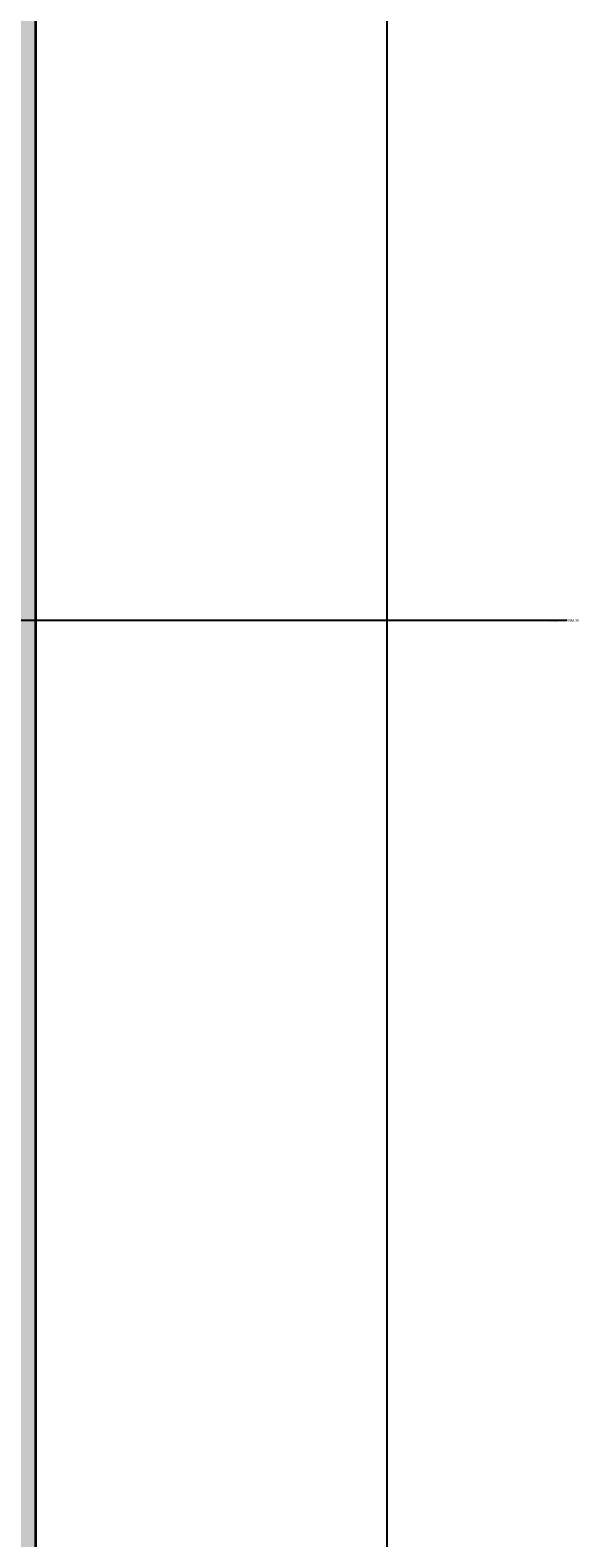
# Model space of a CAD drawing. Units: inches. Extents: x 3024 to 3952, y 1308 to 1863.
# Tile 20 of 29: x 3469 to 3510, y 1449 to 1559. Entities that reach past the tile are written whole.
import ezdxf

# ---------------------------------------------------------------- set-up
doc = ezdxf.new("R2010")
doc.units = ezdxf.units.IN
doc.layers.add('A-ANNO-DIMS', color=2, linetype='Continuous', lineweight=18)
doc.layers.add('A-WALL', color=7, linetype='Continuous', lineweight=35)
doc.layers.add('A-WALL-PATT', color=254, linetype='Continuous', lineweight=13, true_color=0xcecce6)
doc.styles.get("Standard").update_dxf_attribs({"font": 'arial.ttf'})
doc.dimstyles.get("Standard").update_dxf_attribs({"dimtxt": 0.18, "dimasz": 0.18, "dimexe": 0.18, "dimexo": 0.0625, "dimgap": 0.09, "dimtad": 0, "dimtih": 1, "dimtoh": 1, "dimdec": 4, "dimzin": 0, "dimdsep": 46, "dimtxsty": 'Standard', "dimcen": 0.09, "dimadec": 0, "dimazin": 0, "dimtfac": 1, "dimtdec": 4, "dimtofl": 0, "dimtmove": 0, "dimatfit": 3, "dimfxl": 1, "dimtolj": 1, "dimtzin": 0, "dimarcsym": 0})

# ---------------------------------------------------------------- blocks, each defined once
blk = doc.blocks.new('*D37')
at = {"layer": 'A-ANNO-DIMS', "color": 0, "lineweight": -2, "transparency": 16777216}
for p, q in [((3469.83, 1787.61), (3495.72, 1787.61)), ((3495.54, 1787.43), (3495.54, 1567.91)), ((3495.54, 1348.03), (3495.54, 1567.54)), ((3469.83, 1347.85), (3495.72, 1347.85))]:
    blk.add_line(p, q, dxfattribs=at)
at = {"layer": 'A-ANNO-DIMS', "color": 0, "transparency": 16777216}
for points in [[(3495.51, 1787.43), (3495.57, 1787.43), (3495.54, 1787.61)], [(3495.51, 1348.03), (3495.57, 1348.03), (3495.54, 1347.85)]]:
    blk.add_solid(points, dxfattribs=at)
at = {"layer": 'Defpoints', "color": 0, "transparency": 16777216}
for p in [(3469.76, 1787.61), (3495.54, 1787.61), (3469.76, 1347.85)]:
    blk.add_point(p, dxfattribs=at)
at = {"layer": 'A-ANNO-DIMS', "color": 0, "transparency": 16777216, "insert": (3495.54, 1567.73), "char_height": 0.18, "attachment_point": 5}
blk.add_mtext('\\A1;439.8', dxfattribs=at)
blk = doc.blocks.new('*D104')
at = {"layer": 'A-ANNO-DIMS', "color": 0, "lineweight": -2, "transparency": 16777216}
for p, q in [((3360.65, 1515.79), (3360.83, 1515.79)), ((3360.74, 1515.7), (3360.74, 1515.88)), ((3507.36, 1515.79), (3452.55, 1515.79))]:
    blk.add_line(p, q, dxfattribs=at)
at = {"layer": 'A-ANNO-DIMS', "color": 0, "transparency": 16777216}
blk.add_solid([(3452.55, 1515.82), (3452.55, 1515.76), (3452.37, 1515.79)], dxfattribs=at)
at = {"layer": 'Defpoints', "color": 0, "transparency": 16777216}
for p in [(3360.74, 1515.79), (3452.37, 1515.79)]:
    blk.add_point(p, dxfattribs=at)
at = {"layer": 'A-ANNO-DIMS', "color": 0, "transparency": 16777216, "insert": (3507.83, 1515.79), "char_height": 0.18, "attachment_point": 5}
blk.add_mtext('\\A1;R91.64', dxfattribs=at)
blk = doc.blocks.new('*D105')
at = {"layer": 'A-ANNO-DIMS', "color": 0, "lineweight": -2, "transparency": 16777216}
for p, q in [((3370.44, 1515.79), (3370.62, 1515.79)), ((3370.53, 1515.7), (3370.53, 1515.88)), ((3508.74, 1515.79), (3457.09, 1515.79))]:
    blk.add_line(p, q, dxfattribs=at)
at = {"layer": 'A-ANNO-DIMS', "color": 0, "transparency": 16777216}
blk.add_solid([(3457.09, 1515.82), (3457.09, 1515.76), (3456.91, 1515.79)], dxfattribs=at)
at = {"layer": 'Defpoints', "color": 0, "transparency": 16777216}
for p in [(3370.53, 1515.79), (3456.91, 1515.79)]:
    blk.add_point(p, dxfattribs=at)
at = {"layer": 'A-ANNO-DIMS', "color": 0, "transparency": 16777216, "insert": (3509.22, 1515.79), "char_height": 0.18, "attachment_point": 5}
blk.add_mtext('\\A1;R86.38', dxfattribs=at)

msp = doc.modelspace()

# ---------------------------------------------------------------- hatches: boundary and pattern name
at = {"layer": 'A-WALL-PATT'}
h = msp.add_hatch(color=256, dxfattribs=at)
h.dxf.hatch_style = 1
h.paths.add_polyline_path([(3106.764, 1778.6064), (3140.5977, 1778.6064), (3140.5977, 1781.8824), (3140.5977, 1784.6), (3140.5977, 1787.6064), (3097.764, 1787.6064), (3097.764, 1590.213), (3101.04, 1590.213), (3103.7576, 1590.213), (3106.764, 1590.213)])
h.paths.add_polyline_path([(3253.5314, 1781.8824), (3253.5314, 1784.6), (3253.5314, 1787.6064), (3194.6826, 1787.6064), (3194.6826, 1785.0146), (3194.6826, 1784.6), (3194.6826, 1781.8824), (3194.6826, 1778.6064), (3253.5314, 1778.6064)])
h.paths.add_polyline_path([(3333.856, 1782.2838), (3333.856, 1784.7474), (3333.856, 1787.6064), (3272.0523, 1787.6064), (3272.0523, 1785.0146), (3272.0523, 1784.6), (3272.0523, 1781.8824), (3272.0523, 1778.6064), (3333.856, 1778.6064)])
h.paths.add_polyline_path([(3428.8344, 1784.6), (3428.8344, 1787.6064), (3378.3947, 1787.6064), (3378.3947, 1784.7474), (3378.3947, 1782.2838), (3378.3947, 1778.6064), (3428.8344, 1778.6064), (3428.8344, 1781.8824)], flags=17)
h.paths.add_polyline_path([(3469.764, 1787.6064), (3451.9386, 1787.6064), (3451.9386, 1785.0146), (3451.9386, 1784.6), (3451.9386, 1781.8824), (3451.9386, 1778.6064), (3460.764, 1778.6064), (3460.764, 1353.8452), (3277.764, 1353.8452), (3277.764, 1347.8452), (3469.764, 1347.8452), (3469.764, 1353.8452)])
h.paths.add_polyline_path([(3106.764, 1571.6922), (3104.1722, 1571.6922), (3103.7576, 1571.6922), (3101.04, 1571.6922), (3097.764, 1571.6922), (3097.764, 1347.8452), (3148.7271, 1347.8452), (3148.7271, 1351.1212), (3148.7271, 1353.8388), (3148.7271, 1356.8452), (3106.764, 1356.8452)])
h.paths.add_polyline_path([(3277.764, 1532.6064), (3262.7605, 1532.6064), (3262.7605, 1582.9359), (3256.7605, 1582.9359), (3256.7605, 1532.6064), (3244.2116, 1532.6064), (3216.238, 1532.6064), (3216.238, 1527.2064), (3216.238, 1526.6064), (3271.764, 1526.6064), (3271.764, 1356.8452), (3202.812, 1356.8452), (3202.812, 1354.2534), (3202.812, 1353.8388), (3202.812, 1351.1212), (3202.812, 1347.8452), (3277.764, 1347.8452), (3277.764, 1353.8452), (3277.764, 1356.8452)])
h.paths.add_polyline_path([(3180.238, 1532.6064), (3163.0285, 1532.6064), (3163.0285, 1531.1064), (3163.0285, 1526.6064), (3180.243, 1526.6064, -0.00416688), (3180.238, 1527.2064)])
h.paths.add_polyline_path([(3133.0285, 1531.1064, -0.01250587), (3133.066, 1532.6064), (3106.764, 1532.6064), (3106.764, 1526.6064), (3133.0285, 1526.6064)], flags=17)
h.paths.add_polyline_path([(3172.764, 1628.6064), (3166.764, 1628.6064), (3166.764, 1532.6064), (3172.764, 1532.6064)])
h.paths.add_polyline_path([(3232.764, 1649.8972), (3227.364, 1649.8972), (3226.764, 1649.8972), (3226.764, 1634.6064), (3106.764, 1634.6064), (3106.764, 1628.6064), (3232.764, 1628.6064)])

# ---------------------------------------------------------------- linework, layer by layer
at = {"layer": 'A-WALL'}
msp.add_line((3469.764, 1347.8452), (3469.764, 1787.6064), dxfattribs=at)

# ---------------------------------------------------------------- dimensions: what is measured, and where the dimension line sits
at = {"layer": 'A-ANNO-DIMS'}
dim = msp.add_linear_dim(base=(3495.539, 1787.6064), p1=(3469.764, 1347.8452), p2=(3469.764, 1787.6064), angle=90, dimstyle='Standard', override={"dimdec": 1, "dimlfac": 1, "dimrnd": 0, "dimzin": 0, "dimdsep": 46, "dimlunit": 2}, dxfattribs=at)
dim.commit()
dim.dimension.update_dxf_attribs({"geometry": '*D37', "text_midpoint": (3495.539, 1567.7258)})
for center, mpoint, picture, middle in [((3360.7376, 1515.7869), (3452.3735, 1515.787), '*D104', (3507.3551, 1515.7871)), ((3370.5265, 1515.7869), (3456.9101, 1515.787), '*D105', (3508.7402, 1515.7871))]:
    dim = msp.add_radius_dim(center=center, mpoint=mpoint, dimstyle='Standard', override={"dimdec": 2, "dimlfac": 1, "dimrnd": 0, "dimzin": 0, "dimdsep": 46, "dimlunit": 2}, dxfattribs=at)
    dim.commit()
    dim.dimension.update_dxf_attribs({"geometry": picture, "text_midpoint": middle, "dimtype": 164})

doc.saveas('drawing.dxf')
